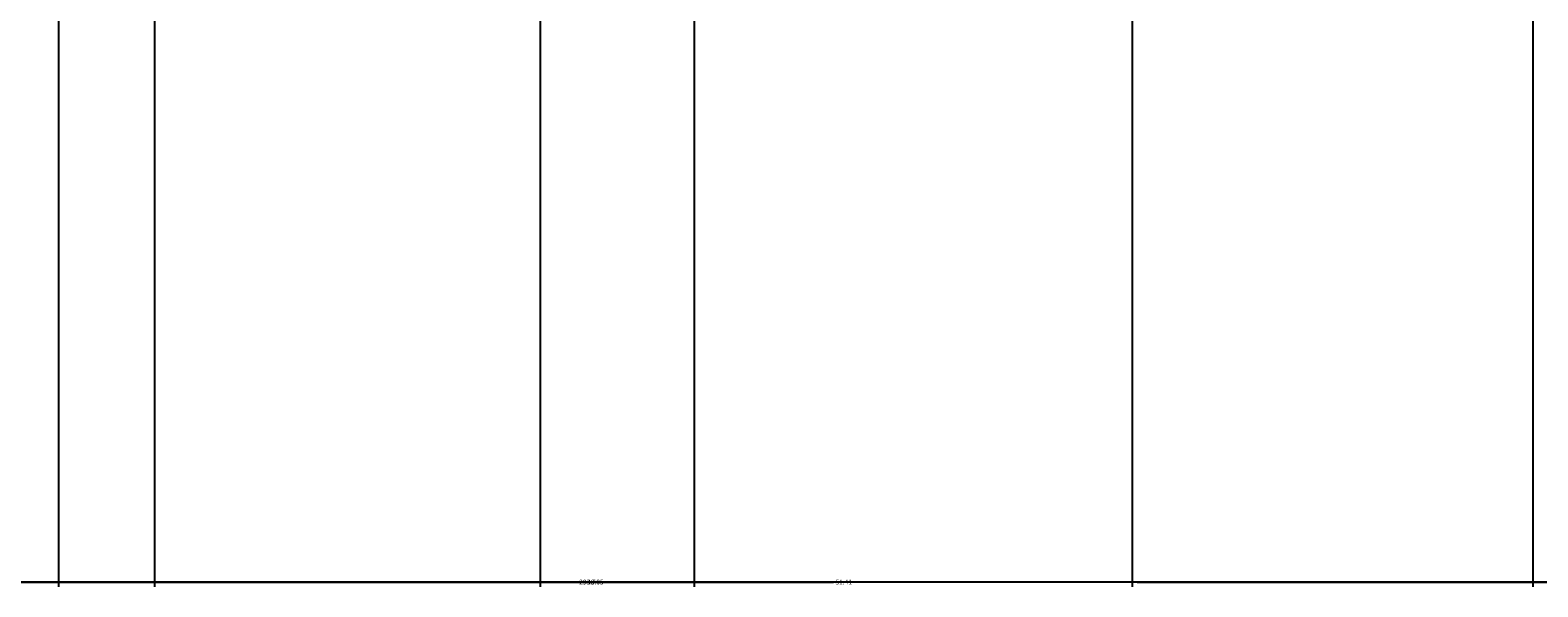
# Model space of a CAD drawing. Units: inches. Extents: x 738 to 1068, y 378 to 757.
# Tile 12 of 41: x 882 to 939, y 378 to 399. Entities that reach past the tile are written whole.
import ezdxf

# ---------------------------------------------------------------- set-up
doc = ezdxf.new("R2010")
doc.units = ezdxf.units.IN
doc.header["$MEASUREMENT"] = 0
doc.layers.add('A-ANNO-DIMS', color=2, linetype='Continuous', lineweight=18)
doc.styles.get("Standard").update_dxf_attribs({"font": 'arial.ttf'})
doc.dimstyles.get("Standard").update_dxf_attribs({"dimtxt": 0.18, "dimasz": 0.18, "dimexe": 0.18, "dimexo": 0.0625, "dimgap": 0.09, "dimtad": 0, "dimtih": 1, "dimtoh": 1, "dimdec": 4, "dimzin": 0, "dimdsep": 46, "dimtxsty": 'Standard', "dimcen": 0.09, "dimadec": 0, "dimazin": 0, "dimtfac": 1, "dimtdec": 4, "dimtofl": 0, "dimtmove": 0, "dimatfit": 3, "dimfxl": 1, "dimtolj": 1, "dimtzin": 0, "dimarcsym": 0})

# ---------------------------------------------------------------- blocks, each defined once
blk = doc.blocks.new('*D17')
at = {"layer": 'A-ANNO-DIMS', "color": 0, "lineweight": -2, "transparency": 16777216}
for p, q in [((756.324, 415.842), (756.324, 378.239)), ((1050.049, 415.919), (1050.049, 378.239)), ((756.504, 378.419), (902.791, 378.419)), ((1049.869, 378.419), (903.582, 378.419))]:
    blk.add_line(p, q, dxfattribs=at)
at = {"layer": 'A-ANNO-DIMS', "color": 0, "transparency": 16777216}
for points in [[(756.504, 378.449), (756.504, 378.389), (756.324, 378.419)], [(1049.869, 378.449), (1049.869, 378.389), (1050.049, 378.419)]]:
    blk.add_solid(points, dxfattribs=at)
at = {"layer": 'Defpoints', "color": 0, "transparency": 16777216}
for p in [(756.324, 415.904), (1050.049, 415.982), (1050.049, 378.419)]:
    blk.add_point(p, dxfattribs=at)
at = {"layer": 'A-ANNO-DIMS', "color": 0, "transparency": 16777216, "insert": (903.186, 378.419), "char_height": 0.18, "attachment_point": 5}
blk.add_mtext('\\A1;293.7', dxfattribs=at)
blk = doc.blocks.new('*D27')
at = {"layer": 'A-ANNO-DIMS', "color": 0, "lineweight": -2, "transparency": 16777216}
for p, q in [((883.457, 646.923), (883.457, 378.239)), ((923.511, 646.923), (923.511, 378.239)), ((883.637, 378.419), (903.086, 378.419)), ((923.331, 378.419), (903.882, 378.419))]:
    blk.add_line(p, q, dxfattribs=at)
at = {"layer": 'A-ANNO-DIMS', "color": 0, "transparency": 16777216}
for points in [[(883.637, 378.449), (883.637, 378.389), (883.457, 378.419)], [(923.331, 378.449), (923.331, 378.389), (923.511, 378.419)]]:
    blk.add_solid(points, dxfattribs=at)
at = {"layer": 'Defpoints', "color": 0, "transparency": 16777216}
for p in [(883.457, 646.985), (923.511, 646.985), (923.511, 378.419)]:
    blk.add_point(p, dxfattribs=at)
at = {"layer": 'A-ANNO-DIMS', "color": 0, "transparency": 16777216, "insert": (903.484, 378.419), "char_height": 0.18, "attachment_point": 5}
blk.add_mtext('\\A1;40.05', dxfattribs=at)
blk = doc.blocks.new('*D28')
at = {"layer": 'A-ANNO-DIMS', "color": 0, "lineweight": -2, "transparency": 16777216}
for p, q in [((923.511, 646.923), (923.511, 378.239)), ((969.439, 646.923), (969.439, 378.239)), ((923.691, 378.419), (946.078, 378.419)), ((969.259, 378.419), (946.872, 378.419))]:
    blk.add_line(p, q, dxfattribs=at)
at = {"layer": 'A-ANNO-DIMS', "color": 0, "transparency": 16777216}
for points in [[(923.691, 378.449), (923.691, 378.389), (923.511, 378.419)], [(969.259, 378.449), (969.259, 378.389), (969.439, 378.419)]]:
    blk.add_solid(points, dxfattribs=at)
at = {"layer": 'Defpoints', "color": 0, "transparency": 16777216}
for p in [(923.511, 646.985), (969.439, 646.985), (969.439, 378.419)]:
    blk.add_point(p, dxfattribs=at)
at = {"layer": 'A-ANNO-DIMS', "color": 0, "transparency": 16777216, "insert": (946.475, 378.419), "char_height": 0.18, "attachment_point": 5}
blk.add_mtext('\\A1;45.93', dxfattribs=at)
blk = doc.blocks.new('*D33')
at = {"layer": 'A-ANNO-DIMS', "color": 0, "lineweight": -2, "transparency": 16777216}
for p, q in [((836.324, 514.624), (836.324, 378.239)), ((907.171, 514.624), (907.171, 378.239)), ((836.504, 378.419), (871.354, 378.419)), ((906.991, 378.419), (872.141, 378.419))]:
    blk.add_line(p, q, dxfattribs=at)
at = {"layer": 'A-ANNO-DIMS', "color": 0, "transparency": 16777216}
for points in [[(836.504, 378.449), (836.504, 378.389), (836.324, 378.419)], [(906.991, 378.449), (906.991, 378.389), (907.171, 378.419)]]:
    blk.add_solid(points, dxfattribs=at)
at = {"layer": 'Defpoints', "color": 0, "transparency": 16777216}
for p in [(836.324, 514.687), (907.171, 514.687), (907.171, 378.419)]:
    blk.add_point(p, dxfattribs=at)
at = {"layer": 'A-ANNO-DIMS', "color": 0, "transparency": 16777216, "insert": (871.748, 378.419), "char_height": 0.18, "attachment_point": 5}
blk.add_mtext('\\A1;70.85', dxfattribs=at)
blk = doc.blocks.new('*D35')
at = {"layer": 'A-ANNO-DIMS', "color": 0, "lineweight": -2, "transparency": 16777216}
for p, q in [((855.932, 686.266), (855.932, 378.239)), ((901.429, 686.267), (901.429, 378.239)), ((856.112, 378.419), (878.352, 378.419)), ((901.249, 378.419), (879.009, 378.419))]:
    blk.add_line(p, q, dxfattribs=at)
at = {"layer": 'A-ANNO-DIMS', "color": 0, "transparency": 16777216}
for points in [[(856.112, 378.449), (856.112, 378.389), (855.932, 378.419)], [(901.249, 378.449), (901.249, 378.389), (901.429, 378.419)]]:
    blk.add_solid(points, dxfattribs=at)
at = {"layer": 'Defpoints', "color": 0, "transparency": 16777216}
for p in [(855.932, 686.329), (901.429, 686.329), (901.429, 378.419)]:
    blk.add_point(p, dxfattribs=at)
at = {"layer": 'A-ANNO-DIMS', "color": 0, "transparency": 16777216, "insert": (878.68, 378.419), "char_height": 0.18, "attachment_point": 5}
blk.add_mtext('\\A1;45.5', dxfattribs=at)
blk = doc.blocks.new('*D38')
at = {"layer": 'A-ANNO-DIMS', "color": 0, "lineweight": -2, "transparency": 16777216}
for p, q in [((781.485, 593.017), (781.485, 378.239)), ((887.04, 593.067), (887.04, 378.239)), ((781.665, 378.419), (833.807, 378.419)), ((886.86, 378.419), (834.718, 378.419))]:
    blk.add_line(p, q, dxfattribs=at)
at = {"layer": 'A-ANNO-DIMS', "color": 0, "transparency": 16777216}
for points in [[(781.665, 378.449), (781.665, 378.389), (781.485, 378.419)], [(886.86, 378.449), (886.86, 378.389), (887.04, 378.419)]]:
    blk.add_solid(points, dxfattribs=at)
at = {"layer": 'Defpoints', "color": 0, "transparency": 16777216}
for p in [(781.485, 593.08), (887.04, 593.13), (887.04, 378.419)]:
    blk.add_point(p, dxfattribs=at)
at = {"layer": 'A-ANNO-DIMS', "color": 0, "transparency": 16777216, "insert": (834.263, 378.419), "char_height": 0.18, "attachment_point": 5}
blk.add_mtext('\\A1;105.56', dxfattribs=at)
blk = doc.blocks.new('*D39')
at = {"layer": 'A-ANNO-DIMS', "color": 0, "lineweight": -2, "transparency": 16777216}
for p, q in [((887.04, 581.418), (887.04, 378.239)), ((938.455, 581.418), (938.455, 378.239)), ((887.22, 378.419), (912.371, 378.419)), ((938.275, 378.419), (913.124, 378.419))]:
    blk.add_line(p, q, dxfattribs=at)
at = {"layer": 'A-ANNO-DIMS', "color": 0, "transparency": 16777216}
for points in [[(887.22, 378.449), (887.22, 378.389), (887.04, 378.419)], [(938.275, 378.449), (938.275, 378.389), (938.455, 378.419)]]:
    blk.add_solid(points, dxfattribs=at)
at = {"layer": 'Defpoints', "color": 0, "transparency": 16777216}
for p in [(887.04, 581.481), (938.455, 581.481), (938.455, 378.419)]:
    blk.add_point(p, dxfattribs=at)
at = {"layer": 'A-ANNO-DIMS', "color": 0, "transparency": 16777216, "insert": (912.748, 378.419), "char_height": 0.18, "attachment_point": 5}
blk.add_mtext('\\A1;51.41', dxfattribs=at)

msp = doc.modelspace()

# ---------------------------------------------------------------- dimensions: what is measured, and where the dimension line sits
at = {"layer": 'A-ANNO-DIMS'}
for base, p1, p2, override, picture, middle in [((901.4286, 378.4191), (855.9323, 686.329), (901.4286, 686.3292), {"dimdec": 1, "dimlfac": 1, "dimrnd": 0, "dimzin": 0, "dimdsep": 46, "dimlunit": 2}, '*D35', (878.6804, 378.4191)), ((923.5105, 378.4191), (883.4574, 646.9853), (923.5105, 646.9853), {"dimdec": 2, "dimlfac": 1, "dimrnd": 0, "dimzin": 0, "dimdsep": 46, "dimlunit": 2}, '*D27', (903.484, 378.4191)), ((969.4395, 378.4191), (923.5105, 646.9853), (969.4395, 646.9853), {"dimdec": 2, "dimlfac": 1, "dimrnd": 0, "dimzin": 0, "dimdsep": 46, "dimlunit": 2}, '*D28', (946.475, 378.4191)), ((887.0404, 378.4191), (781.4846, 593.0796), (887.0404, 593.1296), {"dimdec": 2, "dimlfac": 1, "dimrnd": 0, "dimzin": 0, "dimdsep": 46, "dimlunit": 2}, '*D38', (834.2625, 378.4191)), ((938.455, 378.4191), (887.0404, 581.4808), (938.455, 581.4808), {"dimdec": 2, "dimlfac": 1, "dimrnd": 0, "dimzin": 0, "dimdsep": 46, "dimlunit": 2}, '*D39', (912.7477, 378.4191)), ((907.1708, 378.4191), (836.3244, 514.6866), (907.1708, 514.6866), {"dimdec": 2, "dimlfac": 1, "dimrnd": 0, "dimzin": 0, "dimdsep": 46, "dimlunit": 2}, '*D33', (871.7476, 378.4191)), ((1050.0492, 378.4191), (756.3236, 415.904), (1050.0492, 415.982), {"dimdec": 1, "dimlfac": 1, "dimrnd": 0, "dimzin": 0, "dimdsep": 46, "dimlunit": 2}, '*D17', (903.1864, 378.4191))]:
    dim = msp.add_linear_dim(base=base, p1=p1, p2=p2, dimstyle='Standard', override=override, dxfattribs=at)
    dim.commit()
    dim.dimension.update_dxf_attribs({"geometry": picture, "text_midpoint": middle})

doc.saveas('drawing.dxf')
